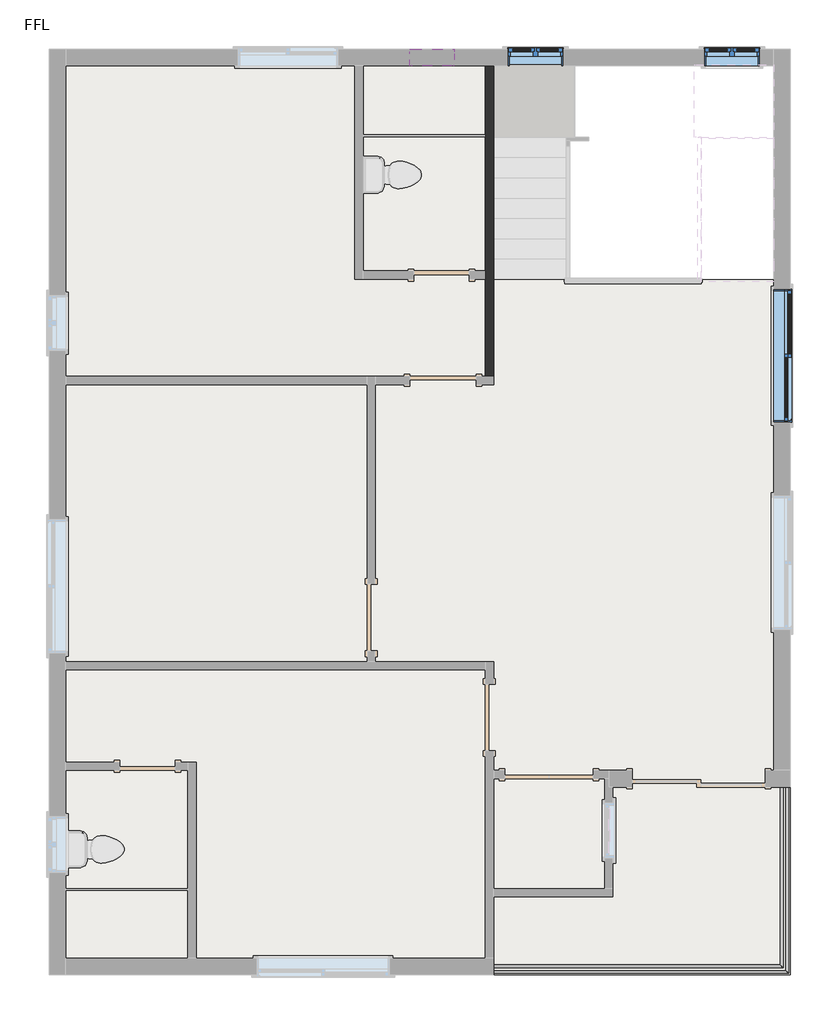
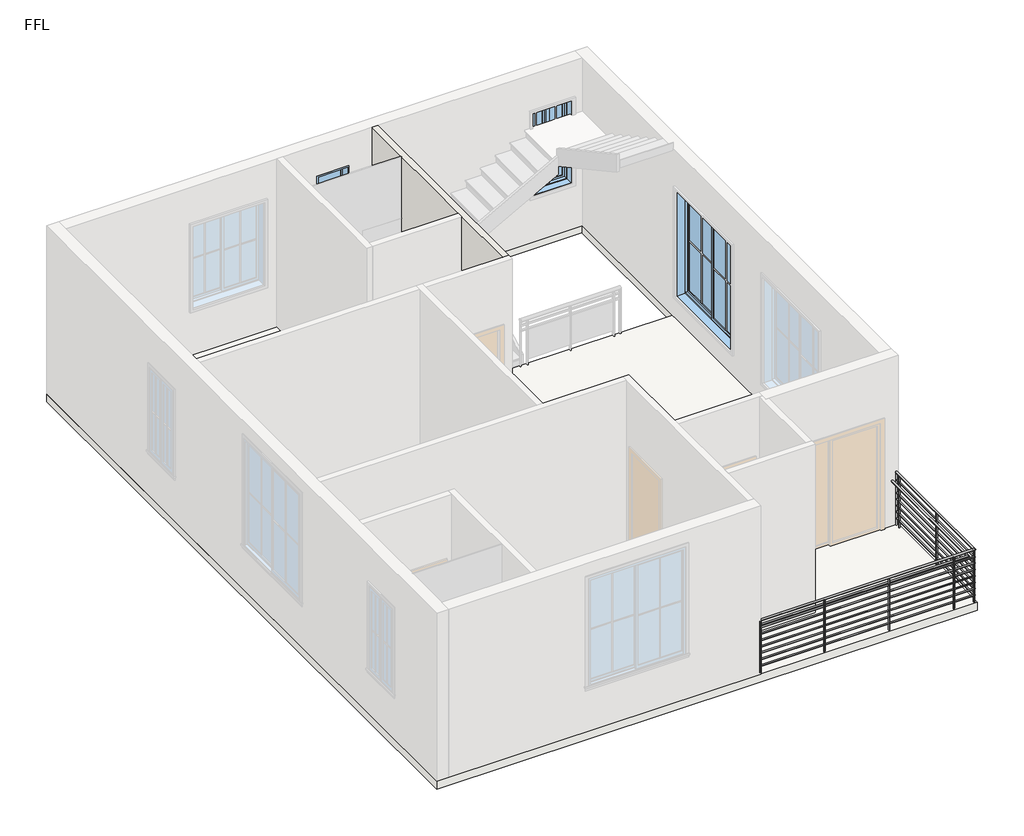
# One storey, part 2 of 3: 4 windows, 1 railing, 1 slab, 1 wall.
"""IFC4 building model written with IfcOpenShell, lengths in millimetres."""

from ifc_helpers import new_model, si_unit, point, frame, frame_2d, origin, place, context, project, spatial, polyline, circle_curve, ellipse_curve, trimmed, segment, composite_curve, outline, extrude, faceted_brep, transform, mapped, element, save
from ifc_brep_helpers import plane_surface, cylinder_surface, advanced_brep
from components import window_80340324, window_9dcce3b5, window_sliding_double_6_x7_726fea71

model = new_model("IFC4")

# Units and contexts
model_context = context("Model", 3, world=origin())
ifc_project = project(units=[si_unit("LENGTHUNIT", "METRE", prefix="MILLI")], contexts=[model_context])

# Site, building, storey
site = spatial("IfcSite", under=ifc_project)
building = spatial("IfcBuilding", under=site)
storey = spatial("IfcBuildingStorey", under=building, Name="FFL", Elevation=3505.2)

# Railing
placement = place(None, origin())
element("IfcRailing", 1, ObjectType="Guardrail - Pipe", at=placement, inside=storey, context=model_context, shape_type="SolidModel", body=[
    advanced_brep(
    [(-7815.600969, -228.1371638, 4400.55), (-7815.600969, -190.0371638, 4400.55), (-3834.150969, -228.1371638, 4400.55), (-3872.250969, -190.0371638, 4400.55), (-3834.150969, 2256.7795268, 4400.55), (-3872.250969, 2256.7795268, 4400.55)],
    [
        (0, 1, circle_curve(frame((-7815.600969, -209.0871638, 4400.55), z_axis=(-1.0, 0.0, 0.0), x_axis=(0.0, 1.0, 0.0)), 19.05)),
        (1, 0, circle_curve(frame((-7815.600969, -209.0871638, 4400.55), z_axis=(-1.0, 0.0, 0.0), x_axis=(0.0, 1.0, 0.0)), 19.05)),
        (0, 2),
        (2, 3, ellipse_curve(frame((-3853.200969, -209.0871638, 4400.55), z_axis=(-0.7071067811865492, -0.7071067811865458, 0.0), x_axis=(-0.7071067811865458, 0.7071067811865491, 0.0)), 26.9407684, 19.05)),
        (3, 1),
        (3, 2, ellipse_curve(frame((-3853.200969, -209.0871638, 4400.55), z_axis=(-0.7071067811865492, -0.7071067811865458, 0.0), x_axis=(-0.7071067811865458, 0.7071067811865491, 0.0)), 26.9407684, 19.05)),
        (4, 5, circle_curve(frame((-3853.200969, 2256.7795268, 4400.55), z_axis=(0.0, 1.0, 0.0), x_axis=(-1.0, 0.0, 0.0)), 19.05)),
        (5, 4, circle_curve(frame((-3853.200969, 2256.7795268, 4400.55), z_axis=(0.0, 1.0, 0.0), x_axis=(-1.0, 0.0, 0.0)), 19.05)),
        (2, 4),
        (5, 3),
    ],
    [
        plane_surface(frame((-7815.600969, -209.0871638, 4419.6), z_axis=(-1.0, 0.0, 0.0), x_axis=(0.0, 1.0, 0.0))),
        cylinder_surface(frame((-7815.600969, -209.0871638, 4400.55), z_axis=(-1.0, 0.0, 0.0), x_axis=(0.0, 1.0, 0.0)), 19.05),
        plane_surface(frame((-3853.200969, 2256.7795268, 4419.6), z_axis=(0.0, 1.0, 0.0), x_axis=(0.0, 0.0, 1.0))),
        cylinder_surface(frame((-3853.200969, -209.0871638, 4400.55), z_axis=(0.0, -1.0, 0.0), x_axis=(-1.0, 0.0, 0.0)), 19.05),
    ],
    [
        (0, [[1, 2]]),
        (1, [[-1, 3, 4, 5]]),
        (1, [[-2, -5, 6, -3]]),
        (2, [[7, 8]]),
        (3, [[-4, 9, -8, 10]]),
        (3, [[-6, -10, -7, -9]]),
    ],
),
    advanced_brep(
    [(-7815.600969, -304.3371638, 4552.95), (-7815.600969, -266.2371638, 4552.95), (-3757.950969, 2256.7795268, 4552.95), (-3796.050969, 2256.7795268, 4552.95), (-3757.950969, -304.3371638, 4552.95), (-3796.050969, -266.2371638, 4552.95)],
    [
        (0, 1, circle_curve(frame((-7815.600969, -285.2871638, 4552.95), z_axis=(-1.0, 0.0, 0.0), x_axis=(0.0, 1.0, 0.0)), 19.05)),
        (1, 0, circle_curve(frame((-7815.600969, -285.2871638, 4552.95), z_axis=(-1.0, 0.0, 0.0), x_axis=(0.0, 1.0, 0.0)), 19.05)),
        (2, 3, circle_curve(frame((-3777.000969, 2256.7795268, 4552.95), z_axis=(0.0, 1.0, 0.0), x_axis=(-1.0, 0.0, 0.0)), 19.05)),
        (3, 2, circle_curve(frame((-3777.000969, 2256.7795268, 4552.95), z_axis=(0.0, 1.0, 0.0), x_axis=(-1.0, 0.0, 0.0)), 19.05)),
        (0, 4),
        (4, 5, ellipse_curve(frame((-3777.000969, -285.2871638, 4552.95), z_axis=(-0.7071067811865492, -0.7071067811865458, 0.0), x_axis=(-0.7071067811865458, 0.7071067811865491, 0.0)), 26.9407684, 19.05)),
        (5, 1),
        (5, 4, ellipse_curve(frame((-3777.000969, -285.2871638, 4552.95), z_axis=(-0.7071067811865492, -0.7071067811865458, 0.0), x_axis=(-0.7071067811865458, 0.7071067811865491, 0.0)), 26.9407684, 19.05)),
        (4, 2),
        (3, 5),
    ],
    [
        plane_surface(frame((-7815.600969, -285.2871638, 4572.0), z_axis=(-1.0, 0.0, 0.0), x_axis=(0.0, 1.0, 0.0))),
        plane_surface(frame((-3777.000969, 2256.7795268, 4572.0), z_axis=(0.0, 1.0, 0.0), x_axis=(0.0, 0.0, 1.0))),
        cylinder_surface(frame((-7815.600969, -285.2871638, 4552.95), z_axis=(-1.0, 0.0, 0.0), x_axis=(0.0, 1.0, 0.0)), 19.05),
        cylinder_surface(frame((-3777.000969, -285.2871638, 4552.95), z_axis=(0.0, -1.0, 0.0), x_axis=(-1.0, 0.0, 0.0)), 19.05),
    ],
    [
        (0, [[1, 2]]),
        (1, [[3, 4]]),
        (2, [[-1, 5, 6, 7]]),
        (2, [[-2, -7, 8, -5]]),
        (3, [[-6, 9, -4, 10]]),
        (3, [[-8, -10, -3, -9]]),
    ],
),
    advanced_brep(
    [(-7815.600969, -272.5871638, 4406.9), (-7815.600969, -297.9871638, 4406.9), (-3789.700969, 2256.7795268, 4406.9), (-3764.300969, 2256.7795268, 4406.9), (-3789.700969, -272.5871638, 4406.9), (-3764.300969, -297.9871638, 4406.9)],
    [
        (0, 1, circle_curve(frame((-7815.600969, -285.2871638, 4406.9), z_axis=(-1.0, 0.0, 0.0), x_axis=(0.0, -1.0, 0.0)), 12.7)),
        (1, 0, circle_curve(frame((-7815.600969, -285.2871638, 4406.9), z_axis=(-1.0, 0.0, 0.0), x_axis=(0.0, -1.0, 0.0)), 12.7)),
        (2, 3, circle_curve(frame((-3777.000969, 2256.7795268, 4406.9), z_axis=(0.0, 1.0, 0.0), x_axis=(1.0, 0.0, 0.0)), 12.7)),
        (3, 2, circle_curve(frame((-3777.000969, 2256.7795268, 4406.9), z_axis=(0.0, 1.0, 0.0), x_axis=(1.0, 0.0, 0.0)), 12.7)),
        (0, 4),
        (4, 5, ellipse_curve(frame((-3777.000969, -285.2871638, 4406.9), z_axis=(-0.7071067811865492, -0.7071067811865458, 0.0), x_axis=(-0.7071067811865458, 0.7071067811865491, 0.0)), 17.9605122, 12.7)),
        (5, 1),
        (5, 4, ellipse_curve(frame((-3777.000969, -285.2871638, 4406.9), z_axis=(-0.7071067811865492, -0.7071067811865458, 0.0), x_axis=(-0.7071067811865458, 0.7071067811865491, 0.0)), 17.9605122, 12.7)),
        (4, 2),
        (3, 5),
    ],
    [
        plane_surface(frame((-7815.600969, -285.2871638, 4419.6), z_axis=(-1.0, 0.0, 0.0), x_axis=(0.0, 1.0, 0.0))),
        plane_surface(frame((-3777.000969, 2256.7795268, 4419.6), z_axis=(0.0, 1.0, 0.0), x_axis=(0.0, 0.0, 1.0))),
        cylinder_surface(frame((-7815.600969, -285.2871638, 4406.9), z_axis=(-1.0, 0.0, 0.0), x_axis=(0.0, -1.0, 0.0)), 12.7),
        cylinder_surface(frame((-3777.000969, -285.2871638, 4406.9), z_axis=(0.0, -1.0, 0.0), x_axis=(1.0, 0.0, 0.0)), 12.7),
    ],
    [
        (0, [[1, 2]]),
        (1, [[3, 4]]),
        (2, [[-1, 5, 6, 7]]),
        (2, [[-2, -7, 8, -5]]),
        (3, [[-6, 9, -4, 10]]),
        (3, [[-8, -10, -3, -9]]),
    ],
),
    advanced_brep(
    [(-7815.600969, -272.5871638, 4279.9), (-7815.600969, -297.9871638, 4279.9), (-3789.700969, 2256.7795268, 4279.9), (-3764.300969, 2256.7795268, 4279.9), (-3789.700969, -272.5871638, 4279.9), (-3764.300969, -297.9871638, 4279.9)],
    [
        (0, 1, circle_curve(frame((-7815.600969, -285.2871638, 4279.9), z_axis=(-1.0, 0.0, 0.0), x_axis=(0.0, -1.0, 0.0)), 12.7)),
        (1, 0, circle_curve(frame((-7815.600969, -285.2871638, 4279.9), z_axis=(-1.0, 0.0, 0.0), x_axis=(0.0, -1.0, 0.0)), 12.7)),
        (2, 3, circle_curve(frame((-3777.000969, 2256.7795268, 4279.9), z_axis=(0.0, 1.0, 0.0), x_axis=(1.0, 0.0, 0.0)), 12.7)),
        (3, 2, circle_curve(frame((-3777.000969, 2256.7795268, 4279.9), z_axis=(0.0, 1.0, 0.0), x_axis=(1.0, 0.0, 0.0)), 12.7)),
        (0, 4),
        (4, 5, ellipse_curve(frame((-3777.000969, -285.2871638, 4279.9), z_axis=(-0.7071067811865492, -0.7071067811865458, 0.0), x_axis=(-0.7071067811865458, 0.7071067811865491, 0.0)), 17.9605122, 12.7)),
        (5, 1),
        (5, 4, ellipse_curve(frame((-3777.000969, -285.2871638, 4279.9), z_axis=(-0.7071067811865492, -0.7071067811865458, 0.0), x_axis=(-0.7071067811865458, 0.7071067811865491, 0.0)), 17.9605122, 12.7)),
        (4, 2),
        (3, 5),
    ],
    [
        plane_surface(frame((-7815.600969, -285.2871638, 4292.6), z_axis=(-1.0, 0.0, 0.0), x_axis=(0.0, 1.0, 0.0))),
        plane_surface(frame((-3777.000969, 2256.7795268, 4292.6), z_axis=(0.0, 1.0, 0.0), x_axis=(0.0, 0.0, 1.0))),
        cylinder_surface(frame((-7815.600969, -285.2871638, 4279.9), z_axis=(-1.0, 0.0, 0.0), x_axis=(0.0, -1.0, 0.0)), 12.7),
        cylinder_surface(frame((-3777.000969, -285.2871638, 4279.9), z_axis=(0.0, -1.0, 0.0), x_axis=(1.0, 0.0, 0.0)), 12.7),
    ],
    [
        (0, [[1, 2]]),
        (1, [[3, 4]]),
        (2, [[-1, 5, 6, 7]]),
        (2, [[-2, -7, 8, -5]]),
        (3, [[-6, 9, -4, 10]]),
        (3, [[-8, -10, -3, -9]]),
    ],
),
    advanced_brep(
    [(-7815.600969, -272.5871638, 4152.9), (-7815.600969, -297.9871638, 4152.9), (-3789.700969, -272.5871638, 4152.9), (-3764.300969, -297.9871638, 4152.9), (-3789.700969, 2256.7795268, 4152.9), (-3764.300969, 2256.7795268, 4152.9)],
    [
        (0, 1, circle_curve(frame((-7815.600969, -285.2871638, 4152.9), z_axis=(-1.0, 0.0, 0.0), x_axis=(0.0, -1.0, 0.0)), 12.7)),
        (1, 0, circle_curve(frame((-7815.600969, -285.2871638, 4152.9), z_axis=(-1.0, 0.0, 0.0), x_axis=(0.0, -1.0, 0.0)), 12.7)),
        (0, 2),
        (2, 3, ellipse_curve(frame((-3777.000969, -285.2871638, 4152.9), z_axis=(-0.7071067811865492, -0.7071067811865458, 0.0), x_axis=(-0.7071067811865458, 0.7071067811865491, 0.0)), 17.9605122, 12.7)),
        (3, 1),
        (3, 2, ellipse_curve(frame((-3777.000969, -285.2871638, 4152.9), z_axis=(-0.7071067811865492, -0.7071067811865458, 0.0), x_axis=(-0.7071067811865458, 0.7071067811865491, 0.0)), 17.9605122, 12.7)),
        (4, 5, circle_curve(frame((-3777.000969, 2256.7795268, 4152.9), z_axis=(0.0, 1.0, 0.0), x_axis=(1.0, 0.0, 0.0)), 12.7)),
        (5, 4, circle_curve(frame((-3777.000969, 2256.7795268, 4152.9), z_axis=(0.0, 1.0, 0.0), x_axis=(1.0, 0.0, 0.0)), 12.7)),
        (2, 4),
        (5, 3),
    ],
    [
        plane_surface(frame((-7815.600969, -285.2871638, 4165.6), z_axis=(-1.0, 0.0, 0.0), x_axis=(0.0, 1.0, 0.0))),
        cylinder_surface(frame((-7815.600969, -285.2871638, 4152.9), z_axis=(-1.0, 0.0, 0.0), x_axis=(0.0, -1.0, 0.0)), 12.7),
        plane_surface(frame((-3777.000969, 2256.7795268, 4165.6), z_axis=(0.0, 1.0, 0.0), x_axis=(0.0, 0.0, 1.0))),
        cylinder_surface(frame((-3777.000969, -285.2871638, 4152.9), z_axis=(0.0, -1.0, 0.0), x_axis=(1.0, 0.0, 0.0)), 12.7),
    ],
    [
        (0, [[1, 2]]),
        (1, [[-1, 3, 4, 5]]),
        (1, [[-2, -5, 6, -3]]),
        (2, [[7, 8]]),
        (3, [[-4, 9, -8, 10]]),
        (3, [[-6, -10, -7, -9]]),
    ],
),
    advanced_brep(
    [(-7815.600969, -272.5871638, 4025.9), (-7815.600969, -297.9871638, 4025.9), (-3789.700969, -272.5871638, 4025.9), (-3764.300969, -297.9871638, 4025.9), (-3789.700969, 2256.7795268, 4025.9), (-3764.300969, 2256.7795268, 4025.9)],
    [
        (0, 1, circle_curve(frame((-7815.600969, -285.2871638, 4025.9), z_axis=(-1.0, 0.0, 0.0), x_axis=(0.0, -1.0, 0.0)), 12.7)),
        (1, 0, circle_curve(frame((-7815.600969, -285.2871638, 4025.9), z_axis=(-1.0, 0.0, 0.0), x_axis=(0.0, -1.0, 0.0)), 12.7)),
        (0, 2),
        (2, 3, ellipse_curve(frame((-3777.000969, -285.2871638, 4025.9), z_axis=(-0.7071067811865492, -0.7071067811865458, 0.0), x_axis=(-0.7071067811865458, 0.7071067811865491, 0.0)), 17.9605122, 12.7)),
        (3, 1),
        (3, 2, ellipse_curve(frame((-3777.000969, -285.2871638, 4025.9), z_axis=(-0.7071067811865492, -0.7071067811865458, 0.0), x_axis=(-0.7071067811865458, 0.7071067811865491, 0.0)), 17.9605122, 12.7)),
        (4, 5, circle_curve(frame((-3777.000969, 2256.7795268, 4025.9), z_axis=(0.0, 1.0, 0.0), x_axis=(1.0, 0.0, 0.0)), 12.7)),
        (5, 4, circle_curve(frame((-3777.000969, 2256.7795268, 4025.9), z_axis=(0.0, 1.0, 0.0), x_axis=(1.0, 0.0, 0.0)), 12.7)),
        (2, 4),
        (5, 3),
    ],
    [
        plane_surface(frame((-7815.600969, -285.2871638, 4038.6), z_axis=(-1.0, 0.0, 0.0), x_axis=(0.0, 1.0, 0.0))),
        cylinder_surface(frame((-7815.600969, -285.2871638, 4025.9), z_axis=(-1.0, 0.0, 0.0), x_axis=(0.0, -1.0, 0.0)), 12.7),
        plane_surface(frame((-3777.000969, 2256.7795268, 4038.6), z_axis=(0.0, 1.0, 0.0), x_axis=(0.0, 0.0, 1.0))),
        cylinder_surface(frame((-3777.000969, -285.2871638, 4025.9), z_axis=(0.0, -1.0, 0.0), x_axis=(1.0, 0.0, 0.0)), 12.7),
    ],
    [
        (0, [[1, 2]]),
        (1, [[-1, 3, 4, 5]]),
        (1, [[-2, -5, 6, -3]]),
        (2, [[7, 8]]),
        (3, [[-4, 9, -8, 10]]),
        (3, [[-6, -10, -7, -9]]),
    ],
),
    advanced_brep(
    [(-7815.600969, -272.5871638, 3898.9), (-7815.600969, -297.9871638, 3898.9), (-3789.700969, -272.5871638, 3898.9), (-3764.300969, -297.9871638, 3898.9), (-3789.700969, 2256.7795268, 3898.9), (-3764.300969, 2256.7795268, 3898.9)],
    [
        (0, 1, circle_curve(frame((-7815.600969, -285.2871638, 3898.9), z_axis=(-1.0, 0.0, 0.0), x_axis=(0.0, -1.0, 0.0)), 12.7)),
        (1, 0, circle_curve(frame((-7815.600969, -285.2871638, 3898.9), z_axis=(-1.0, 0.0, 0.0), x_axis=(0.0, -1.0, 0.0)), 12.7)),
        (0, 2),
        (2, 3, ellipse_curve(frame((-3777.000969, -285.2871638, 3898.9), z_axis=(-0.7071067811865492, -0.7071067811865458, 0.0), x_axis=(-0.7071067811865458, 0.7071067811865491, 0.0)), 17.9605122, 12.7)),
        (3, 1),
        (3, 2, ellipse_curve(frame((-3777.000969, -285.2871638, 3898.9), z_axis=(-0.7071067811865492, -0.7071067811865458, 0.0), x_axis=(-0.7071067811865458, 0.7071067811865491, 0.0)), 17.9605122, 12.7)),
        (4, 5, circle_curve(frame((-3777.000969, 2256.7795268, 3898.9), z_axis=(0.0, 1.0, 0.0), x_axis=(1.0, 0.0, 0.0)), 12.7)),
        (5, 4, circle_curve(frame((-3777.000969, 2256.7795268, 3898.9), z_axis=(0.0, 1.0, 0.0), x_axis=(1.0, 0.0, 0.0)), 12.7)),
        (2, 4),
        (5, 3),
    ],
    [
        plane_surface(frame((-7815.600969, -285.2871638, 3911.6), z_axis=(-1.0, 0.0, 0.0), x_axis=(0.0, 1.0, 0.0))),
        cylinder_surface(frame((-7815.600969, -285.2871638, 3898.9), z_axis=(-1.0, 0.0, 0.0), x_axis=(0.0, -1.0, 0.0)), 12.7),
        plane_surface(frame((-3777.000969, 2256.7795268, 3911.6), z_axis=(0.0, 1.0, 0.0), x_axis=(0.0, 0.0, 1.0))),
        cylinder_surface(frame((-3777.000969, -285.2871638, 3898.9), z_axis=(0.0, -1.0, 0.0), x_axis=(1.0, 0.0, 0.0)), 12.7),
    ],
    [
        (0, [[1, 2]]),
        (1, [[-1, 3, 4, 5]]),
        (1, [[-2, -5, 6, -3]]),
        (2, [[7, 8]]),
        (3, [[-4, 9, -8, 10]]),
        (3, [[-6, -10, -7, -9]]),
    ],
),
    advanced_brep(
    [(-7815.600969, -272.5871638, 3771.9), (-7815.600969, -297.9871638, 3771.9), (-3789.700969, -272.5871638, 3771.9), (-3764.300969, -297.9871638, 3771.9), (-3789.700969, 2256.7795268, 3771.9), (-3764.300969, 2256.7795268, 3771.9)],
    [
        (0, 1, circle_curve(frame((-7815.600969, -285.2871638, 3771.9), z_axis=(-1.0, 0.0, 0.0), x_axis=(0.0, -1.0, 0.0)), 12.7)),
        (1, 0, circle_curve(frame((-7815.600969, -285.2871638, 3771.9), z_axis=(-1.0, 0.0, 0.0), x_axis=(0.0, -1.0, 0.0)), 12.7)),
        (0, 2),
        (2, 3, ellipse_curve(frame((-3777.000969, -285.2871638, 3771.9), z_axis=(-0.7071067811865492, -0.7071067811865458, 0.0), x_axis=(-0.7071067811865458, 0.7071067811865491, 0.0)), 17.9605122, 12.7)),
        (3, 1),
        (3, 2, ellipse_curve(frame((-3777.000969, -285.2871638, 3771.9), z_axis=(-0.7071067811865492, -0.7071067811865458, 0.0), x_axis=(-0.7071067811865458, 0.7071067811865491, 0.0)), 17.9605122, 12.7)),
        (4, 5, circle_curve(frame((-3777.000969, 2256.7795268, 3771.9), z_axis=(0.0, 1.0, 0.0), x_axis=(1.0, 0.0, 0.0)), 12.7)),
        (5, 4, circle_curve(frame((-3777.000969, 2256.7795268, 3771.9), z_axis=(0.0, 1.0, 0.0), x_axis=(1.0, 0.0, 0.0)), 12.7)),
        (2, 4),
        (5, 3),
    ],
    [
        plane_surface(frame((-7815.600969, -285.2871638, 3784.6), z_axis=(-1.0, 0.0, 0.0), x_axis=(0.0, 1.0, 0.0))),
        cylinder_surface(frame((-7815.600969, -285.2871638, 3771.9), z_axis=(-1.0, 0.0, 0.0), x_axis=(0.0, -1.0, 0.0)), 12.7),
        plane_surface(frame((-3777.000969, 2256.7795268, 3784.6), z_axis=(0.0, 1.0, 0.0), x_axis=(0.0, 0.0, 1.0))),
        cylinder_surface(frame((-3777.000969, -285.2871638, 3771.9), z_axis=(0.0, -1.0, 0.0), x_axis=(1.0, 0.0, 0.0)), 12.7),
    ],
    [
        (0, [[1, 2]]),
        (1, [[-1, 3, 4, 5]]),
        (1, [[-2, -5, 6, -3]]),
        (2, [[7, 8]]),
        (3, [[-4, 9, -8, 10]]),
        (3, [[-6, -10, -7, -9]]),
    ],
),
    advanced_brep(
    [(-7815.600969, -272.5871638, 3644.9), (-7815.600969, -297.9871638, 3644.9), (-3789.700969, -272.5871638, 3644.9), (-3764.300969, -297.9871638, 3644.9), (-3789.700969, 2256.7795268, 3644.9), (-3764.300969, 2256.7795268, 3644.9)],
    [
        (0, 1, circle_curve(frame((-7815.600969, -285.2871638, 3644.9), z_axis=(-1.0, 0.0, 0.0), x_axis=(0.0, -1.0, 0.0)), 12.7)),
        (1, 0, circle_curve(frame((-7815.600969, -285.2871638, 3644.9), z_axis=(-1.0, 0.0, 0.0), x_axis=(0.0, -1.0, 0.0)), 12.7)),
        (0, 2),
        (2, 3, ellipse_curve(frame((-3777.000969, -285.2871638, 3644.9), z_axis=(-0.7071067811865492, -0.7071067811865458, 0.0), x_axis=(-0.7071067811865458, 0.7071067811865491, 0.0)), 17.9605122, 12.7)),
        (3, 1),
        (3, 2, ellipse_curve(frame((-3777.000969, -285.2871638, 3644.9), z_axis=(-0.7071067811865492, -0.7071067811865458, 0.0), x_axis=(-0.7071067811865458, 0.7071067811865491, 0.0)), 17.9605122, 12.7)),
        (4, 5, circle_curve(frame((-3777.000969, 2256.7795268, 3644.9), z_axis=(0.0, 1.0, 0.0), x_axis=(1.0, 0.0, 0.0)), 12.7)),
        (5, 4, circle_curve(frame((-3777.000969, 2256.7795268, 3644.9), z_axis=(0.0, 1.0, 0.0), x_axis=(1.0, 0.0, 0.0)), 12.7)),
        (2, 4),
        (5, 3),
    ],
    [
        plane_surface(frame((-7815.600969, -285.2871638, 3657.6), z_axis=(-1.0, 0.0, 0.0), x_axis=(0.0, 1.0, 0.0))),
        cylinder_surface(frame((-7815.600969, -285.2871638, 3644.9), z_axis=(-1.0, 0.0, 0.0), x_axis=(0.0, -1.0, 0.0)), 12.7),
        plane_surface(frame((-3777.000969, 2256.7795268, 3657.6), z_axis=(0.0, 1.0, 0.0), x_axis=(0.0, 0.0, 1.0))),
        cylinder_surface(frame((-3777.000969, -285.2871638, 3644.9), z_axis=(0.0, -1.0, 0.0), x_axis=(1.0, 0.0, 0.0)), 12.7),
    ],
    [
        (0, [[1, 2]]),
        (1, [[-1, 3, 4, 5]]),
        (1, [[-2, -5, 6, -3]]),
        (2, [[7, 8]]),
        (3, [[-4, 9, -8, 10]]),
        (3, [[-6, -10, -7, -9]]),
    ],
),
    extrude(outline(composite_curve([segment(trimmed(circle_curve(frame_2d((-3777.000969, 2153.1128362)), 12.7), [point((-3789.700969, 2153.1128362))], [point((-3764.300969, 2153.1128362))], False, "CARTESIAN"), True, "CONTINUOUS"), segment(trimmed(circle_curve(frame_2d((-3777.000969, 2153.1128362)), 12.7), [point((-3764.300969, 2153.1128362))], [point((-3789.700969, 2153.1128362))], False, "CARTESIAN"), True, "CONTINUOUS")], self_intersect=False)), frame((0.0, 0.0, 3505.2), z_axis=(0.0, 0.0, 1.0), x_axis=(1.0, 0.0, 0.0)), (0.0, 0.0, 1.0), 1028.7),
    extrude(outline(composite_curve([segment(trimmed(circle_curve(frame_2d((-3777.000969, 933.9128362)), 12.7), [point((-3789.700969, 933.9128362))], [point((-3764.300969, 933.9128362))], False, "CARTESIAN"), True, "CONTINUOUS"), segment(trimmed(circle_curve(frame_2d((-3777.000969, 933.9128362)), 12.7), [point((-3764.300969, 933.9128362))], [point((-3789.700969, 933.9128362))], False, "CARTESIAN"), True, "CONTINUOUS")], self_intersect=False)), frame((0.0, 0.0, 3505.2), z_axis=(0.0, 0.0, 1.0), x_axis=(1.0, 0.0, 0.0)), (0.0, 0.0, 1.0), 1028.7),
    extrude(outline(composite_curve([segment(trimmed(circle_curve(frame_2d((-4158.000969, -285.2871638)), 12.7), [point((-4158.000969, -272.5871638))], [point((-4158.000969, -297.9871638))], False, "CARTESIAN"), True, "CONTINUOUS"), segment(trimmed(circle_curve(frame_2d((-4158.000969, -285.2871638)), 12.7), [point((-4158.000969, -297.9871638))], [point((-4158.000969, -272.5871638))], False, "CARTESIAN"), True, "CONTINUOUS")], self_intersect=False)), frame((0.0, 0.0, 3505.2), z_axis=(0.0, 0.0, 1.0), x_axis=(1.0, 0.0, 0.0)), (0.0, 0.0, 1.0), 1028.7),
    extrude(outline(composite_curve([segment(trimmed(circle_curve(frame_2d((-5377.200969, -285.2871638)), 12.7), [point((-5377.200969, -272.5871638))], [point((-5377.200969, -297.9871638))], False, "CARTESIAN"), True, "CONTINUOUS"), segment(trimmed(circle_curve(frame_2d((-5377.200969, -285.2871638)), 12.7), [point((-5377.200969, -297.9871638))], [point((-5377.200969, -272.5871638))], False, "CARTESIAN"), True, "CONTINUOUS")], self_intersect=False)), frame((0.0, 0.0, 3505.2), z_axis=(0.0, 0.0, 1.0), x_axis=(1.0, 0.0, 0.0)), (0.0, 0.0, 1.0), 1028.7),
    extrude(outline(composite_curve([segment(trimmed(circle_curve(frame_2d((-6596.400969, -285.2871638)), 12.7), [point((-6596.400969, -272.5871638))], [point((-6596.400969, -297.9871638))], False, "CARTESIAN"), True, "CONTINUOUS"), segment(trimmed(circle_curve(frame_2d((-6596.400969, -285.2871638)), 12.7), [point((-6596.400969, -297.9871638))], [point((-6596.400969, -272.5871638))], False, "CARTESIAN"), True, "CONTINUOUS")], self_intersect=False)), frame((0.0, 0.0, 3505.2), z_axis=(0.0, 0.0, 1.0), x_axis=(1.0, 0.0, 0.0)), (0.0, 0.0, 1.0), 1028.7),
    extrude(outline(composite_curve([segment(trimmed(circle_curve(frame_2d((-3777.000969, -285.2871638)), 12.7), [point((-3777.000969, -272.5871638))], [point((-3777.000969, -297.9871638))], False, "CARTESIAN"), True, "CONTINUOUS"), segment(trimmed(circle_curve(frame_2d((-3777.000969, -285.2871638)), 12.7), [point((-3777.000969, -297.9871638))], [point((-3777.000969, -272.5871638))], False, "CARTESIAN"), True, "CONTINUOUS")], self_intersect=False)), frame((0.0, 0.0, 3505.2), z_axis=(0.0, 0.0, 1.0), x_axis=(1.0, 0.0, 0.0)), (0.0, 0.0, 1.0), 1028.7),
    extrude(outline(composite_curve([segment(trimmed(circle_curve(frame_2d((-3777.000969, 2244.0795268)), 12.7), [point((-3789.700969, 2244.0795268))], [point((-3764.300969, 2244.0795268))], False, "CARTESIAN"), True, "CONTINUOUS"), segment(trimmed(circle_curve(frame_2d((-3777.000969, 2244.0795268)), 12.7), [point((-3764.300969, 2244.0795268))], [point((-3789.700969, 2244.0795268))], False, "CARTESIAN"), True, "CONTINUOUS")], self_intersect=False)), frame((0.0, 0.0, 3505.2), z_axis=(0.0, 0.0, 1.0), x_axis=(1.0, 0.0, 0.0)), (0.0, 0.0, 1.0), 1028.7),
    extrude(outline(composite_curve([segment(trimmed(circle_curve(frame_2d((-7802.900969, -285.2871638)), 12.7), [point((-7802.900969, -272.5871638))], [point((-7802.900969, -297.9871638))], False, "CARTESIAN"), True, "CONTINUOUS"), segment(trimmed(circle_curve(frame_2d((-7802.900969, -285.2871638)), 12.7), [point((-7802.900969, -297.9871638))], [point((-7802.900969, -272.5871638))], False, "CARTESIAN"), True, "CONTINUOUS")], self_intersect=False)), frame((0.0, 0.0, 3505.2), z_axis=(0.0, 0.0, 1.0), x_axis=(1.0, 0.0, 0.0)), (0.0, 0.0, 1.0), 1028.7),
])

# Slab
element("IfcSlab", 2, ObjectType="6\"", at=placement, inside=storey, context=model_context, shape_type="SweptSolid", body=[
    extrude(outline(polyline([(-3735.7257748, 12402.0128362), (-3735.7257748, -323.3871638), (-13924.3002526, -323.3871638), (-13924.3002526, 12402.0128362), (-3735.7257748, 12402.0128362)]), holes=[polyline([(-3961.1502526, 12192.4628362), (-7815.6002526, 12192.4628362), (-7815.6002526, 9239.7128362), (-3961.1502526, 9239.7128362), (-3961.1502526, 12192.4628362)])]), frame((0.0, 0.0, 3352.8), z_axis=(0.0, 0.0, 1.0), x_axis=(1.0, 0.0, 0.0)), (0.0, 0.0, 1.0), 152.4),
])

# Wall
element("IfcWall", 3, ObjectType="5\"", at=placement, inside=storey, context=model_context, shape_type="Brep", body=[
    faceted_brep([(-7815.6002526, 7906.2128362, 3505.2), (-7815.6002526, 12173.4128362, 3505.2), (-7815.6002526, 12173.4128362, 6858.0), (-7815.6002526, 7906.2128362, 6858.0), (-7929.9002526, 7906.2128362, 3505.2), (-7929.9002526, 7906.2128362, 6858.0), (-7929.9002526, 9239.7128699, 6858.0), (-7929.9002526, 9354.0128699, 6858.0), (-7929.9002526, 12173.4128362, 6858.0), (-7929.9002526, 12173.4128362, 3505.2), (-7929.9002526, 9354.0128699, 3505.2), (-7929.9002526, 9239.7128699, 3505.2)], [[[0, 1, 2, 3]], [[4, 5, 6, 7, 8, 9, 10, 11]], [[1, 0, 4, 11, 10, 9]], [[3, 2, 8, 7, 6, 5]], [[0, 3, 5, 4]], [[2, 1, 9, 8]]]),
])

# Windows
window_shape = window_80340324(model_context)
element("IfcWindow", 4, ObjectType="Fixed : 24\" x 24\"", at=placement, inside=storey, context=model_context, shape_type="MappedRepresentation", body=[
    mapped(window_shape, transform((-8622.0502526, 12287.7128362, 4724.4), x_axis=(1.0, 0.0, 0.0), y_axis=(0.0, 1.0, 0.0), z_axis=(0.0, 0.0, 1.0))),
])
window_2_shape = window_9dcce3b5(model_context)
element("IfcWindow", 5, ObjectType="Window-Casement-Double : 2'-6\" X 5'-6\"", at=placement, inside=storey, context=model_context, shape_type="MappedRepresentation", body=[
    mapped(window_2_shape, transform((-7237.7502526, 12287.7128362, 2590.8), x_axis=(1.0, 0.0, 0.0), y_axis=(0.0, 1.0, 0.0), z_axis=(0.0, 0.0, 1.0))),
])
element("IfcWindow", 6, ObjectType="Window-Casement-Double : 2'-6\" X 5'-6\"", at=placement, inside=storey, context=model_context, shape_type="MappedRepresentation", body=[
    mapped(window_2_shape, transform((-4535.8257748, 12287.7128362, 3505.2), x_axis=(1.0, 0.0, 0.0), y_axis=(0.0, 1.0, 0.0), z_axis=(0.0, 0.0, 1.0))),
])
window_sliding_double_6_x7_shape = window_sliding_double_6_x7_726fea71(model_context)
element("IfcWindow", 7, ObjectType="Window-Sliding-Double : 6'X7'", at=placement, inside=storey, context=model_context, shape_type="MappedRepresentation", body=[
    mapped(window_sliding_double_6_x7_shape, transform((-3846.2157748, 8187.6795268, 3048.0), x_axis=(0.0, -1.0, 0.0), y_axis=(1.0, 0.0, 0.0), z_axis=(0.0, 0.0, 1.0))),
])

save(model, "model.ifc")

# Revit data of these elements
# Type "Guardrail - Pipe"
#   Assembly Code = "C2010400"
#   built-in parameter 1008612 = 0.0416667 (stored number, unit not read)
#   built-in parameter 1008611 = 0.0833333 (stored number, unit not read)
#   built-in parameter 1008609 = 4 (stored number, unit not read)
#   built-in parameter 1008604 = 0.166667 (stored number, unit not read)
#   built-in parameter 1008603 = 0.166667 (stored number, unit not read)
#   Railing Height = 3' - 6"
#   built-in parameter 1008630 = 2
#   built-in parameter 1008610 = 1
#   built-in parameter 1008605 = 1
#   built-in parameter 1008618 = Baluster - Round : 1"
# Type "6\""
#   Assembly Code = "B1010"
#   Function = 0
#   Layers, outside or top first: 0' - 6" "Gypsum Wall Board" (function 1)
# Type "5\""
#   Assembly Code = "B2010"
#   Layers, outside or top first: 0' - 4 1/2" "Gypsum Wall Board" (function 1)
# Type "Fixed : 24\" x 24\""
#   Type Mark = "3"
#   Construction Type Id = "GSP4R"
#   Assembly Code = "B2020100"
#   Analytic Construction = "1/8 in Pilkington single glazing"
#   Visual Light Transmittance = 0.9
#   Solar Heat Gain Coefficient = 0.78
#   Heat Transfer Coefficient (U) = 0.6496 BTU/(h·ft²·°F)
#   Height = 2' - 0"
#   Default Sill Height = 3' - 0"
#   Width = 2' - 0"
#   Window Inset = 0' - 0 3/4"
#   Define Thermal Properties by = 1
#   Define Thermal Properties by = 1
#   Glass Pane Material = Glass
#   Sash Material = Sash
#   Wall Closure = (empty or 0)
# Type "Window-Casement-Double : 2'-6\" X 5'-6\""
#   Type Mark = "21"
#   Fire Rating = "0.5h"
#   Assembly Code = "B2020100"
#   Analytic Construction = "Double glazing - domestic"
#   Frame Extension [instance default] = 0' - 0 1/4"
#   Window Inset [instance default] = 0' - 0"
#   Wall Thickness [instance default] = 0' - 6"
#   Interior Wall Closure [instance default] = 0' - 2 1/4"
#   Half Width = 1' - 3"
#   Visual Light Transmittance = 0.81
#   Thermal Resistance (R) = 1.8146 (h·ft²·°F)/BTU
#   Solar Heat Gain Coefficient = 0.76
#   Rough Width = 2' - 6 1/2"
#   Rough Height = 5' - 6 1/2"
#   Height = 5' - 6"
#   Heat Transfer Coefficient (U) = 0.5511 BTU/(h·ft²·°F)
#   Exterior Wall Closure [instance default] = 0' - 1 1/4"
#   Extension Jamb [instance default] = 0' - 2 1/4"
#   Default Sill Height = 3' - 0"
#   Width = 2' - 6"
#   Muntin Visibility = yes
#   Interior Trim Visibility [instance default] = yes
#   Exterior Trim Visibility [instance default] = yes
#   Extension Jamb Visibility [instance default] = yes
#   Interior Trim Material = Wood - Stained
#   Muntin Pattern = Muntin Pattern_2x2 : Muntin Pattern_2x2
#   Interior Trim = Trim-Window-Interior-Flat : Picture Frame
#   Interior Frame Material = Wood - Stained
#   Glass Panel Material = Glass
#   Exterior Trim Material = Clad - White
#   Exterior Trim = Trim-Window-Exterior-Flat : with Sill
#   Exterior Frame Material = Clad - White
#   Wall Closure = (empty or 0)
# Type "Window-Sliding-Double : 6'X7'"
#   Type Mark = "19"
#   Fire Rating = "0.5h"
#   Assembly Code = "B2020100"
#   Analytic Construction = "Double glazing - domestic"
#   Window Inset [instance default] = 0' - 0"
#   Wall Thickness [instance default] = 0' - 6"
#   Visual Light Transmittance = 0.81
#   Thermal Resistance (R) = 1.8146 (h·ft²·°F)/BTU
#   Solar Heat Gain Coefficient = 0.76
#   Muntin Width = 2' - 8 5/8"
#   Muntin Height = 6' - 6 1/4"
#   Interior Wall Closure [instance default] = 0' - 2 3/4"
#   Heat Transfer Coefficient (U) = 0.5511 BTU/(h·ft²·°F)
#   Frame Extension [instance default] = 0' - 0 1/4"
#   Exterior Wall Closure [instance default] = 0' - 1 1/4"
#   Rough Width = 6' - 0 1/2"
#   Rough Height = 7' - 0 1/2"
#   Height = 7' - 0"
#   Extension Jamb [instance default] = 0' - 2 3/4"
#   Default Sill Height = 3' - 0"
#   Width = 6' - 0"
#   Interior Trim Visibility [instance default] = yes
#   Indicator Visibility [instance default] = yes
#   Exterior Trim Visibility [instance default] = yes
#   Muntin Visibility = yes
#   Extension Jamb Visibility [instance default] = yes
#   Muntin Pattern = Muntin Pattern_2x2 : Muntin Pattern_2x2
#   Interior Trim Material = Wood - Stained
#   Interior Trim = Trim-Window-Interior-Flat : Picture Frame
#   Interior Frame Material = Wood - Stained
#   Glass Panel Material = Glass
#   Exterior Trim Material = Clad - White
#   Exterior Trim = Trim-Window-Exterior-Flat : with Sill
#   Exterior Frame Material = Clad - White
#   Wall Closure = (empty or 0)
# Element 1 (IfcRailing, "Guardrail - Pipe")
#   Phase Created = New Construction
# Element 2 (IfcSlab, "6\"")
#   Height Offset From Level = 0' - 0"
#   Phase Created = New Construction
#   Materials on its faces: "Gypsum Wall Board"
# Element 3 (IfcWall, "5\"")
#   Top Offset = 0' - 0"
#   Base Offset = 0' - 0"
#   Unconnected Height = 11' - 0"
#   wall height = 11' - 0"
#   Phase Created = New Construction
#   Base Constraint = FFL
#   Materials on its faces: "Gypsum Wall Board"
# Element 4 (IfcWindow, "Fixed : 24\" x 24\"")
#   Mark = "19"
#   Phase Created = New Construction
#   Materials on its faces: "Sash", "Glass"
# Element 5 (IfcWindow, "Window-Casement-Double : 2'-6\" X 5'-6\"")
#   Mark = "20"
#   Window Inset = 0' - 0"
#   Interior Wall Closure = 0' - 2 1/4"
#   Frame Extension = 0' - 0 1/4"
#   Exterior Wall Closure = 0' - 1 1/4"
#   Interior Trim Visibility = yes
#   Exterior Trim Visibility = yes
#   Phase Created = New Construction
#   Materials on its faces: "Wood - Stained", "Glass", "Clad - White"
# Element 6 (IfcWindow, "Window-Casement-Double : 2'-6\" X 5'-6\"")
#   Mark = "21"
#   Window Inset = 0' - 0"
#   Interior Wall Closure = 0' - 2 1/4"
#   Frame Extension = 0' - 0 1/4"
#   Exterior Wall Closure = 0' - 1 1/4"
#   Interior Trim Visibility = yes
#   Exterior Trim Visibility = yes
#   Phase Created = New Construction
#   Materials on its faces: "Wood - Stained", "Glass", "Clad - White"
# Element 7 (IfcWindow, "Window-Sliding-Double : 6'X7'")
#   Mark = "15"
#   Window Inset = 0' - 0"
#   Interior Wall Closure = 0' - 2 3/4"
#   Frame Extension = 0' - 0 1/4"
#   Exterior Wall Closure = 0' - 1 1/4"
#   Interior Trim Visibility = yes
#   Indicator Visibility = yes
#   Exterior Trim Visibility = yes
#   Phase Created = New Construction
#   Materials on its faces: "Wood - Stained", "Glass", "Clad - White"
# Materials
#   "Gypsum Wall Board": class "Generic", colour RGB 228 228 228, transparency 0, Description = "Gypsum Wall Board", Cost = 0
#   "Glass": class "Glass", colour RGB 0 128 192, transparency 0.75, Description = "Soda Lime Glass", Cost = 0
#   "Sash": class "Wood", colour RGB 224 178 126, transparency 0, Cost = 0
#   "Wood - Stained": class "Wood", colour RGB 224 178 126, transparency 0, Cost = 0
#   "Clad - White": class "Wood", colour RGB 242 242 238, transparency 0, Cost = 0
